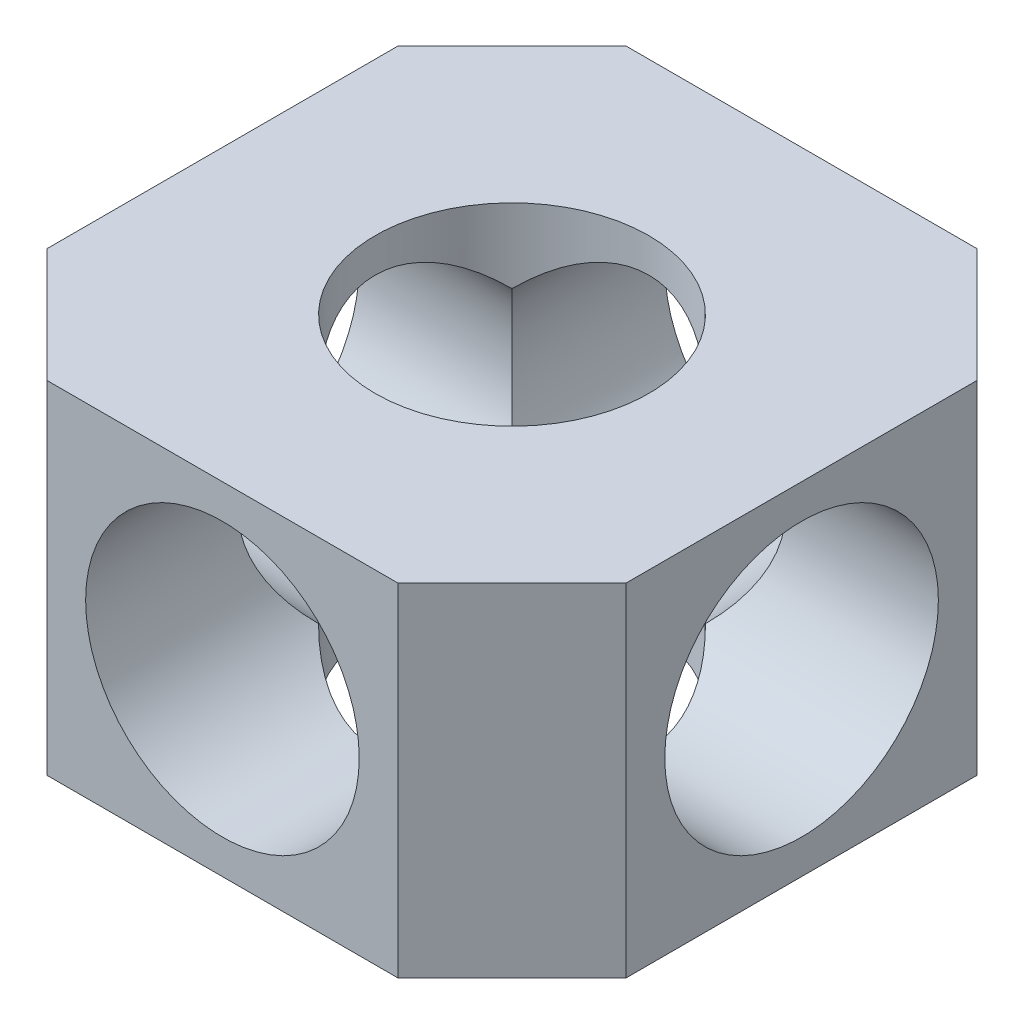
SolidWorks part; units mm, degrees
material "Plain Carbon Steel"
ref_plane "Front Plane" through (0, 0, 0) normal (0, 0, 1) x (1, 0, 0)
ref_plane "Top Plane" through (0, 0, 0) normal (0, 1, 0) x (1, 0, 0)
ref_plane "Right Plane" through (0, 0, 0) normal (1, 0, 0) x (0, 0, -1)
sketch "Base Square Sketch" plane through (0, 0, 0) normal (0, 1, 0) x (1, 0, 0)
  line L1 (12.7, 0) -> (12.7, 12.7)
  line L2 (12.7, 12.7) -> (-12.7, 12.7)
  line L3 (-12.7, 12.7) -> (-12.7, -12.7)
  line L4 (-12.7, -12.7) -> (12.7, -12.7)
  line L5 (12.7, -12.7) -> (12.7, 0)
  dimension "D1" = 25.4
  dimension "D2" = 25.4
  dimension "D3" = 12.7
  dimension "D4" = 12.7
extrude "Base Block" add sketch "Base Square Sketch" along normal blind 15
chamfer "Corner Chamfer 1" distance 5 angle 45 1 edges at (12.7, 7.5, 12.7)
chamfer "Corner Chamfer 2" distance 5 angle 45 1 edges at (12.7, 7.5, -12.7)
chamfer "Corner Chamfer 3" distance 5 angle 45 1 edges at (-12.7, 7.5, -12.7)
chamfer "Corner Chamfer 4" distance 5 angle 45 1 edges at (-12.7, 7.5, 12.7)
sketch "Side Hole A Sketch" plane through (0, 0, -12.7) normal (0, 0, -1) x (-1, 0, 0)
  line L0 (-7.7, 15) -> (-7.7, 0) construction
  circle A0 centre (0, 7.5) radius 6
  dimension "D1" = 12
  dimension "D2" = 7.5
  dimension "D3" = 7.7
extrude "Side Hole A Ø12" cut sketch "Side Hole A Sketch" against normal blind 36
sketch "Side Hole B Sketch" plane through (12.7, 0, 0) normal (1, 0, 0) x (0, 0, -1)
  line L0 (-7.7, 0) -> (7.7, 0) construction
  line L3 (-7.7, 15) -> (-7.7, 0) construction
  circle A0 centre (0, 7.5) radius 6
  dimension "D1" = 12
  dimension "D2" = 7.5
  dimension "D3" = 7.7
extrude "Side Hole B Ø12" cut sketch "Side Hole B Sketch" against normal blind 36
sketch "Vertical Bore Sketch" plane through (0, 15, 0) normal (0, 1, 0) x (1, 0, 0)
  circle A0 centre (0, 0) radius 6
  dimension "D1" = 12
extrude "Vertical Bore Ø12" cut sketch "Vertical Bore Sketch" against normal blind 36
